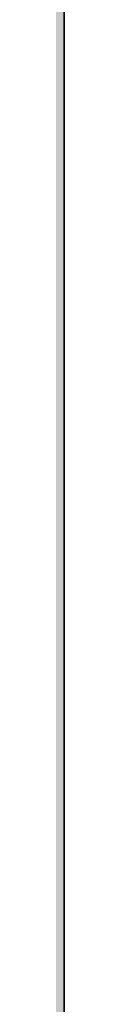
# Model space of a CAD drawing. Units: inches. Extents: x 2091 to 2899, y 967 to 2217.
# Tile 62 of 256: x 2212.1436 to 2212.1436, y 1100.1654 to 1100.4988. Entities that reach past the tile are written whole.
import ezdxf

# ---------------------------------------------------------------- set-up
doc = ezdxf.new("R2010")
doc.units = ezdxf.units.IN
doc.layers.add('A-WALL', color=7, linetype='Continuous', lineweight=35)
doc.layers.add('A-WALL-PATT', color=141, linetype='Continuous', lineweight=13, true_color=0xadddf7)

msp = doc.modelspace()

# ---------------------------------------------------------------- hatches: boundary and pattern name
at = {"layer": 'A-WALL-PATT'}
h = msp.add_hatch(color=256, dxfattribs=at)
h.dxf.hatch_style = 1
h.paths.add_polyline_path([(2212.1436, 1941.41906), (2387.6436, 1941.41906), (2387.6436, 1824.41906), (2392.1436, 1824.41906), (2392.1436, 1941.41906), (2609.6436, 1941.41906), (2609.6436, 1825.91906), (2614.1436, 1825.91906), (2614.1436, 1941.41906), (2794.1436, 1941.41906), (2794.1436, 1928.76217), (2803.1436, 1928.76217), (2803.1436, 2050.91906), (2203.1436, 2050.91906), (2203.1436, 1900.75786), (2212.1436, 1900.75786)])
h.paths.add_polyline_path([(2212.1436, 1945.91906), (2212.1436, 2041.91906), (2794.1436, 2041.91906), (2794.1436, 1945.91906), (2402.24824, 1945.91906), (2401.10243, 1945.77583), (2398.70243, 1945.77583)], flags=16)
h.paths.add_polyline_path([(2230.22986, 1948.06279), (2227.34986, 1949.50279), (2225.90986, 1951.90279), (2223.98986, 1952.86279), (2223.02986, 1955.26279), (2222.06986, 1959.58279), (2222.06986, 1963.42279), (2223.02986, 1965.66279), (2223.98986, 1965.34279), (2225.58591, 1963.86075), (2226.91153, 1964.95726), (2226.94886, 1965.93879), (2227.77832, 1966.95214), (2228.19992, 1968.8787), (2230.70986, 1964.86279), (2233.58986, 1966.30279), (2233.60731, 1966.33187), (2233.77266, 1964.9382), (2234.6338, 1963.67647), (2235.02986, 1963.90279), (2236.28203, 1965.57236), (2235.98986, 1962.94279), (2237.95451, 1957.54), (2238.38986, 1957.90279), (2239.21586, 1960.30579), (2238.65457, 1966.38496), (2238.69279, 1966.43807), (2238.84058, 1967.49971), (2238.78029, 1967.68749), (2238.88054, 1967.78676), (2238.66686, 1966.25179), (2239.21586, 1960.30579), (2238.38986, 1957.90279), (2236.94986, 1956.70279), (2234.54986, 1949.98279)], flags=0)
h.paths.add_polyline_path([(2278.01197, 1948.06279), (2276.49643, 1947.87335), (2275.84983, 1947.68861), (2274.65197, 1947.10279)], flags=0)
h.paths.add_polyline_path([(2269.85197, 1955.74279), (2268.27618, 1956.62933), (2270.8673, 1956.3484), (2269.37197, 1958.14279), (2268.71496, 1959.19233), (2270.56983, 1958.72861), (2268.58073, 1961.90609), (2270.81197, 1960.89188), (2270.81197, 1963.42279), (2271.39331, 1964.77926), (2270.29176, 1966.1562), (2271.77197, 1965.66279), (2272.14139, 1966.52476), (2273.92983, 1965.92861), (2275.63039, 1968.0543), (2276.33194, 1966.72186), (2276.52043, 1966.95214), (2276.94203, 1968.8787), (2277.73429, 1967.61108), (2278.13989, 1969.46452), (2279.65912, 1967.03374), (2280.41197, 1966.78279), (2280.9493, 1967.58879), (2281.60983, 1967.36861), (2282.13327, 1968.15376), (2282.34924, 1966.33344), (2282.34985, 1966.33259), (2283.40755, 1968.09542), (2283.71263, 1965.52402), (2284.32022, 1964.63379), (2284.51181, 1964.88924), (2284.23497, 1965.70479), (2284.50047, 1967.31896), (2284.90794, 1965.41742), (2285.39631, 1966.06858), (2285.43283, 1966.29061), (2285.47334, 1966.17128), (2286.35392, 1967.34539), (2286.22201, 1966.15817), (2287.66349, 1968.08015), (2287.71397, 1968.44279), (2288.4816, 1969.01668), (2288.57399, 1968.7289), (2288.91746, 1969.06904), (2288.60683, 1966.83761), (2288.92873, 1963.35131), (2288.93497, 1963.35679), (2288.92973, 1963.34042), (2289.01528, 1962.41387), (2290.11122, 1963.87513), (2290.13283, 1963.94261), (2290.21767, 1964.01706), (2290.11122, 1963.87513), (2289.15583, 1960.89161), (2288.59404, 1959.25723), (2288.57197, 1959.10279), (2289.53197, 1960.54279), (2290.01197, 1962.46279), (2290.19184, 1962.64266), (2289.76983, 1959.68861), (2286.88983, 1957.28861), (2284.48983, 1950.56861), (2283.31466, 1950.04631), (2283.29197, 1949.98279), (2280.29006, 1948.64861), (2281.12983, 1948.64861), (2282.56983, 1948.16861), (2283.20473, 1948.06279), (2278.97197, 1948.06279), (2276.09197, 1949.50279), (2274.65197, 1951.90279), (2272.73197, 1952.86279)], flags=0)
h.paths.add_polyline_path([(2271.15887, 1958.02177), (2272.96983, 1955.84861), (2272.00983, 1960.16861), (2272.00983, 1964.00861), (2272.62443, 1965.44266), (2274.32802, 1963.86075), (2275.65365, 1964.95726), (2275.63774, 1964.53909), (2277.41223, 1966.00689), (2277.03297, 1965.15679), (2276.82992, 1964.9756), (2276.76601, 1963.29501), (2277.44964, 1962.66022), (2279.45197, 1964.86279), (2282.33197, 1966.30279), (2283.52983, 1966.88861), (2283.29451, 1966.77095), (2283.91299, 1963.8847), (2284.89925, 1964.44827), (2284.73197, 1962.94279), (2286.69662, 1957.54), (2287.13197, 1957.90279), (2287.54191, 1959.09539), (2287.7794, 1958.44231), (2285.68274, 1956.6951), (2285.8765, 1959.79534), (2284.73197, 1962.94279), (2284.89925, 1964.44827), (2283.91299, 1963.8847), (2284.22383, 1962.43412), (2283.42436, 1963.60548), (2281.60983, 1962.56861), (2281.12983, 1960.16861), (2282.08983, 1956.32861), (2283.04983, 1952.96861), (2282.56983, 1950.56861), (2280.16983, 1948.64861), (2279.88332, 1948.79187), (2278.97197, 1948.06279), (2278.97197, 1949.02279), (2278.67231, 1949.39737), (2277.28983, 1950.08861), (2275.84983, 1952.48861), (2273.92983, 1953.44861), (2272.48983, 1954.88861), (2271.92165, 1954.88861), (2271.77197, 1955.26279)], flags=0)
h.paths.add_polyline_path([(2311.99415, 1955.74279), (2312.06272, 1955.67422), (2312.0551, 1955.7085)], flags=0)
h.paths.add_polyline_path([(2331.95615, 1963.95179), (2333.39615, 1965.39179), (2331.07715, 1963.35679), (2330.9986, 1963.11152)], flags=0)
h.paths.add_polyline_path([(2310.55415, 1954.30279), (2307.03981, 1956.27994), (2310.7629, 1955.87628), (2312.47415, 1953.82279), (2313.43415, 1951.42279), (2315.35415, 1950.46279), (2316.79415, 1948.06279), (2317.46615, 1947.72679), (2319.36869, 1947.96461), (2317.75415, 1949.98279), (2317.56953, 1950.61048), (2316.79415, 1951.90279), (2314.87415, 1952.86279), (2313.91415, 1955.26279), (2311.51415, 1958.14279), (2309.37549, 1961.55917), (2311.51415, 1960.33708), (2311.51415, 1961.98279), (2310.60467, 1963.11963), (2311.72661, 1962.47853), (2312.41833, 1964.09256), (2312.25596, 1964.29552), (2313.19415, 1963.98279), (2313.91415, 1965.66279), (2314.64678, 1965.41858), (2315.35415, 1966.30279), (2316.79415, 1967.74279), (2316.15744, 1966.9469), (2317.03411, 1965.28186), (2317.2226, 1965.51214), (2317.77705, 1968.04577), (2318.47411, 1966.72186), (2318.6626, 1966.95214), (2319.0842, 1968.8787), (2321.20705, 1965.48215), (2322.16142, 1966.9137), (2322.55415, 1966.78279), (2322.78599, 1967.13056), (2322.88165, 1966.32429), (2323.31204, 1965.72174), (2323.65129, 1965.89136), (2324.3965, 1967.13338), (2324.65694, 1964.9382), (2324.97199, 1964.47661), (2325.38728, 1967.0015), (2325.94081, 1964.41835), (2327.22893, 1966.13584), (2327.16632, 1965.57236), (2328.05914, 1966.76278), (2328.22458, 1966.24749), (2329.66797, 1967.67691), (2329.66458, 1967.68749), (2329.76482, 1967.78676), (2329.55115, 1966.25179), (2330.10015, 1960.30579), (2329.33281, 1958.07347), (2329.31306, 1957.93523), (2329.63415, 1958.20279), (2330.23415, 1959.10279), (2330.71415, 1961.02279), (2331.03415, 1961.34279), (2330.71415, 1959.10279), (2329.63415, 1958.20279), (2329.27415, 1957.66279), (2327.71211, 1956.3611), (2325.43415, 1949.98279), (2324.33377, 1949.49374), (2323.99415, 1948.54279), (2319.67415, 1946.62279), (2316.79415, 1948.06279), (2315.35415, 1950.46279), (2313.43415, 1951.42279)], flags=0)
h.paths.add_polyline_path([(2321.33568, 1947.95202), (2321.11415, 1948.06279), (2321.11415, 1949.02279), (2319.19415, 1951.42279), (2316.79415, 1959.58279), (2316.66324, 1959.58279), (2315.35415, 1958.14279), (2314.39415, 1958.14279), (2313.1483, 1958.70908), (2312.95415, 1959.58279), (2312.95415, 1960.89188), (2315.83415, 1959.58279), (2316.66324, 1959.58279), (2317.31471, 1960.29941), (2315.0302, 1962.42075), (2316.35582, 1963.51726), (2316.37234, 1963.95162), (2316.4702, 1963.86075), (2317.79582, 1964.95726), (2317.75522, 1963.88969), (2319.17515, 1965.15679), (2319.49841, 1965.88137), (2321.11415, 1965.34279), (2323.23589, 1962.37236), (2325.68635, 1963.77262), (2325.54279, 1962.48058), (2325.19878, 1963.49401), (2324.47851, 1963.08243), (2324.92601, 1960.99412), (2324.07809, 1962.23647), (2322.41479, 1961.28602), (2322.07415, 1959.58279), (2323.03415, 1955.74279), (2323.99415, 1952.38279), (2323.51415, 1949.98279), (2322.14272, 1948.88565), (2322.07415, 1948.54279)], flags=0)
h.paths.add_polyline_path([(2320.20748, 1963.33746), (2320.15415, 1963.42279), (2320.39415, 1963.54279)], flags=0)
h.paths.add_polyline_path([(2353.85053, 1965.8105), (2354.03053, 1965.7505), (2354.33053, 1966.4505), (2354.33053, 1966.9305)], flags=0)
h.paths.add_polyline_path([(2359.02058, 1969.02641), (2359.09838, 1968.90193), (2359.23353, 1969.5195), (2359.23353, 1969.9995)], flags=0)
h.paths.add_polyline_path([(2358.25669, 1966.68167), (2357.9836, 1966.34803), (2358.21127, 1966.14617), (2358.41049, 1966.38957)], flags=0)
h.paths.add_polyline_path([(2357.76847, 1966.05878), (2357.7322, 1965.10497), (2357.75105, 1965.12056), (2357.76953, 1965.6065), (2357.76953, 1966.05784)], flags=0)
h.paths.add_polyline_path([(2359.11153, 1965.3045), (2359.11153, 1964.8245), (2359.84453, 1966.4675), (2359.84453, 1966.9475)], flags=0)
h.paths.add_polyline_path([(2360.22368, 1966.62145), (2360.69853, 1969.3625), (2360.69853, 1969.8425), (2360.21053, 1967.0255), (2360.21053, 1966.6425)], flags=0)
h.paths.add_polyline_path([(2363.45053, 1967.8905), (2363.45053, 1968.3705), (2362.49053, 1966.9305), (2362.65604, 1966.69878)], flags=0)
h.paths.add_polyline_path([(2364.47552, 1966.07883), (2365.85053, 1968.3705), (2365.85053, 1968.8505), (2364.42798, 1966.47958)], flags=0)
h.paths.add_polyline_path([(2366.31353, 1965.8525), (2366.36671, 1965.69583), (2366.80253, 1968.3455), (2366.80253, 1968.8255)], flags=0)
h.paths.add_polyline_path([(2367.16531, 1965.80354), (2367.29053, 1966.9305), (2367.29053, 1967.4105), (2367.1027, 1965.72007)], flags=0)
h.paths.add_polyline_path([(2370.03653, 1959.9735), (2371.01353, 1963.0245), (2371.01353, 1963.5045), (2370.03653, 1960.4535)], flags=0)
h.paths.add_polyline_path([(2371.61053, 1960.2105), (2372.57053, 1961.6505), (2372.57053, 1962.1305), (2371.80253, 1960.9785)], flags=0)
h.paths.add_polyline_path([(2350.87367, 1956.00509), (2351.93053, 1955.8905), (2354.49053, 1953.3305), (2353.85053, 1954.9305), (2351.45053, 1957.8105), (2347.93553, 1963.4255), (2347.93553, 1963.9055), (2351.45053, 1958.2905), (2353.70507, 1955.58505), (2352.89053, 1959.2505), (2352.89053, 1959.7305), (2352.89053, 1961.92479), (2356.73053, 1959.7305), (2358.45447, 1961.62684), (2354.81053, 1965.0105), (2355.03086, 1965.28591), (2358.69109, 1961.88712), (2361.53053, 1965.0105), (2364.3765, 1966.43348), (2364.52439, 1965.18691), (2365.45447, 1963.82418), (2365.88107, 1964.06795), (2365.37053, 1966.4505), (2365.37053, 1966.9305), (2366.81053, 1960.2105), (2366.81053, 1959.7305), (2366.38871, 1952.98141), (2367.77053, 1956.8505), (2368.64123, 1957.57608), (2366.81053, 1962.6105), (2366.81053, 1963.0905), (2368.77518, 1957.68771), (2369.21053, 1958.0505), (2370.00159, 1960.35187), (2369.47523, 1966.05267), (2369.51346, 1966.10578), (2369.51417, 1966.11091), (2369.47523, 1966.53267), (2369.51346, 1966.58578), (2369.61463, 1967.31259), (2369.18253, 1968.6585), (2369.18253, 1969.1385), (2369.60096, 1967.83519), (2369.7012, 1967.93447), (2369.71795, 1968.05474), (2370.14518, 1968.37414), (2369.77871, 1968.01122), (2369.7012, 1967.45447), (2370.46816, 1968.214), (2369.67494, 1967.26577), (2369.51417, 1966.11091), (2370.03653, 1960.4535), (2370.03653, 1959.9735), (2369.44176, 1958.24319), (2370.65053, 1959.2505), (2371.04582, 1962.01756), (2371.13053, 1962.1305), (2370.65053, 1958.7705), (2367.77053, 1956.3705), (2365.37053, 1949.6505), (2362.0791, 1948.18764), (2363.45053, 1947.7305), (2361.05053, 1947.7305), (2360.09053, 1947.7305), (2357.10386, 1947.35717), (2360.09053, 1948.2105), (2358.17053, 1949.1705), (2356.73053, 1951.5705), (2354.81053, 1952.5305), (2351.93053, 1955.4105)], flags=0)
h.paths.add_polyline_path([(2361.05053, 1948.6905), (2359.13053, 1951.0905), (2356.73053, 1959.2505), (2355.77053, 1959.2505), (2352.89053, 1960.55959), (2352.89053, 1961.44479), (2355.89053, 1959.7305), (2356.73053, 1959.7305), (2356.83719, 1959.36783), (2361.53053, 1964.5305), (2363.24842, 1965.38945), (2364.92531, 1963.0418), (2362.49053, 1961.6505), (2362.06386, 1959.51717), (2362.97053, 1955.8905), (2363.93053, 1952.5305), (2363.93053, 1952.0505), (2363.45053, 1949.6505), (2361.05053, 1947.7305)], flags=0)
h.paths.add_polyline_path([(2359.13053, 1951.5705), (2359.29053, 1951.3705), (2361.05053, 1954.4505), (2361.05053, 1954.9305)], flags=0)
h.paths.add_polyline_path([(2357.21953, 1966.5455), (2356.79253, 1968.8145), (2356.79253, 1969.2945), (2357.21953, 1967.0255)], flags=0)
h.paths.add_polyline_path([(2361.05053, 1954.4505), (2361.53053, 1958.7705), (2361.53053, 1959.2505), (2361.05053, 1954.9305)], flags=0)
h.paths.add_polyline_path([(2402.54829, 1948.48608), (2402.30243, 1948.41583), (2402.59043, 1948.41583)], flags=0)
h.paths.add_polyline_path([(2394.14243, 1956.09583), (2395.68505, 1954.55321), (2396.7205, 1953.97068), (2396.06243, 1955.61583), (2395.24138, 1956.6011), (2395.8789, 1956.44171), (2395.10243, 1959.93583), (2395.10243, 1963.77583), (2396.06243, 1966.01583), (2397.02243, 1965.69583), (2398.61848, 1964.21379), (2399.94411, 1965.3103), (2399.98143, 1966.29183), (2400.81089, 1967.30518), (2401.23249, 1969.23174), (2403.53795, 1965.54301), (2403.94198, 1967.38932), (2404.70243, 1967.13583), (2405.46033, 1966.07478), (2406.62243, 1966.65583), (2406.63988, 1966.68491), (2406.80523, 1965.29124), (2406.92569, 1965.11475), (2407.34243, 1964.97583), (2407.87433, 1965.77367), (2408.1691, 1964.39805), (2409.31461, 1965.9254), (2409.21746, 1965.05105), (2409.44523, 1963.13124), (2410.30637, 1961.86951), (2410.70243, 1962.09583), (2411.44227, 1963.08228), (2411.16543, 1963.89783), (2411.61643, 1966.63976), (2411.72536, 1966.79111), (2411.87315, 1967.85275), (2411.81286, 1968.04053), (2411.91311, 1968.1398), (2411.69943, 1966.60483), (2412.24843, 1960.65883), (2413.22543, 1963.70983), (2414.3779, 1964.72116), (2414.51315, 1965.69275), (2414.45286, 1965.88053), (2414.55311, 1965.9798), (2414.3779, 1964.72116), (2414.51982, 1964.8457), (2414.36536, 1964.63111), (2414.33943, 1964.44483), (2414.88843, 1958.49883), (2414.06243, 1956.09583), (2412.62243, 1954.89583), (2410.17137, 1948.03285), (2410.01672, 1948.0844), (2405.90243, 1946.25583), (2405.90243, 1947.21583), (2405.20425, 1948.08856), (2404.22243, 1948.41583), (2403.26243, 1948.41583), (2400.38243, 1949.85583), (2399.66243, 1951.05583), (2397.98243, 1952.73583), (2397.02243, 1953.21583), (2395.68505, 1954.55321), (2392.65678, 1956.25691)], flags=0)
h.paths.add_polyline_path([(2409.08565, 1964.40744), (2409.13036, 1964.27572), (2409.26243, 1964.49583)], flags=0)
h.paths.add_polyline_path([(2397.74243, 1961.61583), (2398.70243, 1963.85583), (2399.66243, 1963.53583), (2401.42656, 1965.74099), (2401.79142, 1966.5588), (2402.07143, 1965.07083), (2402.83551, 1964.39337), (2403.2624, 1964.9149), (2403.33812, 1964.77109), (2402.61552, 1963.97622), (2402.49861, 1960.90224), (2403.543, 1959.93245), (2404.4132, 1960.88968), (2404.70243, 1962.33583), (2407.91635, 1964.17235), (2409.52021, 1961.92694), (2410.98708, 1957.89304), (2411.42243, 1958.25583), (2412.04796, 1960.07562), (2412.41034, 1959.07909), (2411.67562, 1958.46682), (2411.66243, 1958.25583), (2411.62607, 1958.42553), (2409.98243, 1957.05583), (2407.58243, 1950.33583), (2403.26243, 1948.41583), (2403.26243, 1949.37583), (2401.34243, 1951.77583), (2399.41651, 1958.32398), (2397.74243, 1959.08492), (2397.74243, 1959.97012), (2397.10243, 1960.33583), (2397.74243, 1960.04492)], flags=0)
h.paths.add_polyline_path([(2405.90243, 1952.97583), (2405.95043, 1953.40783), (2406.01672, 1953.17583)], flags=0)
h.paths.add_polyline_path([(2449.81778, 1967.11401), (2449.75232, 1967.13583), (2449.7937, 1967.0779)], flags=0)
h.paths.add_polyline_path([(2451.6977, 1966.61812), (2451.74089, 1966.69012), (2451.69205, 1966.6657)], flags=0)
h.paths.add_polyline_path([(2454.34363, 1965.73757), (2455.75232, 1967.61583), (2455.99232, 1968.09583), (2454.3645, 1965.9254)], flags=0)
h.paths.add_polyline_path([(2457.54732, 1968.86383), (2457.78732, 1969.34383), (2457.05432, 1968.79583), (2457.00762, 1968.46034)], flags=0)
h.paths.add_polyline_path([(2456.92178, 1967.85666), (2456.80224, 1968.22902), (2456.723, 1967.6598)], flags=0)
h.paths.add_polyline_path([(2457.30232, 1967.37683), (2457.54232, 1967.85683), (2456.81032, 1966.83983), (2456.74052, 1966.70022), (2456.74902, 1966.60811)], flags=0)
h.paths.add_polyline_path([(2458.27532, 1963.70983), (2458.15534, 1963.33515), (2460.35432, 1965.26483), (2460.59432, 1965.74483)], flags=0)
h.paths.add_polyline_path([(2458.39232, 1962.81583), (2458.36409, 1962.61819), (2459.59232, 1964.25583), (2459.83232, 1964.73583)], flags=0)
h.paths.add_polyline_path([(2459.35232, 1962.81583), (2459.27232, 1962.49583), (2460.07232, 1963.29583), (2460.31232, 1963.77583)], flags=0)
h.paths.add_polyline_path([(2458.68032, 1960.60783), (2458.63232, 1960.41583), (2459.59232, 1961.85583), (2459.83232, 1962.33583)], flags=0)
h.paths.add_polyline_path([(2437.83817, 1956.24265), (2439.19232, 1956.09583), (2441.35232, 1953.93583), (2440.87232, 1955.13583), (2438.47232, 1958.01583), (2438.07156, 1958.65602), (2438.71232, 1958.49583), (2440.6396, 1956.18311), (2439.91232, 1959.45583), (2439.91232, 1963.29583), (2441.35232, 1966.65583), (2441.59232, 1967.13583), (2441.11232, 1966.01583), (2442.07232, 1965.69583), (2443.98899, 1968.09167), (2444.24132, 1966.75083), (2444.9168, 1966.15192), (2445.67657, 1967.08014), (2446.25532, 1969.72483), (2446.49532, 1970.20483), (2446.28238, 1969.23174), (2447.36267, 1967.50327), (2447.72032, 1969.56783), (2447.96032, 1970.04783), (2447.48548, 1967.30678), (2448.79232, 1965.21583), (2448.47232, 1964.86383), (2448.55232, 1964.73583), (2451.45205, 1966.1857), (2451.61512, 1964.81124), (2452.30792, 1963.79617), (2453.23451, 1964.32565), (2454.07232, 1960.41583), (2453.62869, 1953.31765), (2454.79232, 1956.57583), (2455.03232, 1957.05583), (2455.71884, 1957.62793), (2453.83232, 1962.81583), (2453.94097, 1963.79362), (2453.33532, 1965.57783), (2453.82432, 1968.55083), (2454.06432, 1969.03083), (2453.57532, 1966.05783), (2454.04033, 1964.68792), (2453.83232, 1962.81583), (2455.71884, 1957.62793), (2456.36721, 1958.16824), (2457.05832, 1960.17883), (2457.29832, 1960.65883), (2456.47232, 1958.25583), (2457.71773, 1959.29367), (2457.67232, 1958.97583), (2454.88995, 1956.65719), (2453.61414, 1953.08492), (2453.59232, 1952.73583), (2453.35232, 1952.25583), (2453.3596, 1952.3722), (2452.63232, 1950.33583), (2452.39232, 1949.85583), (2449.20375, 1948.43869), (2450.71232, 1947.93583), (2448.07232, 1947.93583), (2447.11232, 1947.93583), (2444.55232, 1947.61583), (2447.1996, 1948.3722), (2445.19232, 1949.37583), (2443.75232, 1951.77583), (2441.83232, 1952.73583), (2438.95232, 1955.61583)], flags=0)
h.paths.add_polyline_path([(2443.99232, 1959.93583), (2444.04032, 1959.77263), (2444.12155, 1959.86199)], flags=0)
h.paths.add_polyline_path([(2442.91232, 1959.93583), (2443.03232, 1959.93583), (2442.44566, 1960.2025)], flags=0)
h.paths.add_polyline_path([(2444.98294, 1965.01968), (2445.27932, 1965.26483), (2445.51932, 1965.74483), (2444.994, 1965.3103)], flags=0)
h.paths.add_polyline_path([(2446.13332, 1965.02983), (2446.33037, 1965.4715), (2444.97032, 1964.25783), (2444.73032, 1963.77783)], flags=0)
h.paths.add_polyline_path([(2442.79232, 1959.45583), (2443.75232, 1959.45583), (2446.15232, 1951.29583), (2446.41232, 1951.75083), (2446.39232, 1951.77583), (2448.0806, 1954.73032), (2448.55232, 1958.97583), (2441.83232, 1965.21583), (2442.15495, 1965.61911), (2448.79232, 1959.45583), (2448.31232, 1955.13583), (2448.07232, 1954.65583), (2446.41232, 1951.75083), (2448.31232, 1949.37583), (2448.31232, 1948.41583), (2450.54089, 1950.19869), (2450.95232, 1952.25583), (2449.99232, 1955.61583), (2449.03232, 1959.45583), (2449.51232, 1961.85583), (2449.75232, 1962.33583), (2449.6749, 1961.94874), (2452.99451, 1963.84565), (2453.06441, 1963.51941), (2452.88461, 1963.78285), (2449.6749, 1961.94874), (2449.27232, 1959.93583), (2450.23232, 1956.09583), (2451.19232, 1952.73583), (2450.71232, 1950.33583), (2450.47232, 1949.85583), (2448.07232, 1947.93583), (2448.07232, 1948.53583), (2445.43232, 1949.85583), (2443.99232, 1952.25583), (2442.07232, 1953.21583), (2441.11232, 1955.61583), (2440.15232, 1959.93583), (2440.15232, 1960.65583)], flags=0)
h.paths.add_polyline_path([(2456.69232, 1966.98583), (2457.60832, 1968.08083), (2457.84832, 1968.56083), (2456.93232, 1967.46583)], flags=0)
h.paths.add_polyline_path([(2489.89657, 1966.58024), (2489.94295, 1966.18935), (2490.74749, 1967.53025), (2491.31912, 1968.95116)], flags=0)
h.paths.add_polyline_path([(2473.56247, 1956.40713), (2477.13998, 1956.01926), (2476.95533, 1956.24083), (2475.10805, 1957.28011), (2476.34749, 1956.97025), (2475.1869, 1958.82422), (2476.91912, 1958.39116), (2475.41164, 1960.79927), (2477.78749, 1959.71934), (2477.78749, 1962.25025), (2477.6374, 1962.43786), (2477.82255, 1962.33206), (2478.35912, 1963.58406), (2478.35912, 1963.67116), (2477.32435, 1964.96463), (2478.71483, 1964.50114), (2479.31912, 1965.91116), (2480.27912, 1965.59116), (2481.78397, 1967.47221), (2482.11649, 1965.70525), (2482.88056, 1965.02778), (2483.20931, 1965.42941), (2483.22017, 1965.71509), (2483.07594, 1965.98902), (2483.71176, 1966.76581), (2484.13049, 1968.67925), (2484.70212, 1970.10016), (2484.48918, 1969.12707), (2486.5029, 1965.90511), (2487.38749, 1965.61025), (2488.15342, 1966.75914), (2488.71702, 1965.97011), (2489.20009, 1966.21164), (2489.33067, 1965.11099), (2490.3939, 1963.62246), (2490.66077, 1963.77496), (2490.49391, 1964.55364), (2490.92306, 1963.92484), (2491.31912, 1964.15116), (2491.33339, 1964.17018), (2491.21049, 1964.53225), (2491.28176, 1964.96554), (2491.42579, 1964.29338), (2494.07648, 1967.82763), (2494.49792, 1966.51494), (2494.59817, 1966.61422), (2494.68949, 1967.27025), (2495.10675, 1967.5822), (2495.12984, 1967.74807), (2495.06955, 1967.93585), (2495.1698, 1968.03513), (2495.03178, 1967.04363), (2495.75382, 1967.75868), (2494.98205, 1966.68644), (2494.95612, 1966.50016), (2495.47902, 1960.83685), (2495.91049, 1962.18425), (2496.48212, 1963.60516), (2496.07269, 1962.32659), (2496.7689, 1962.93754), (2496.59912, 1962.71116), (2496.11912, 1959.35116), (2496.73287, 1960.27179), (2496.98749, 1961.29025), (2497.55912, 1962.71116), (2497.07912, 1960.79116), (2496.50749, 1959.37025), (2495.54749, 1957.93025), (2492.75884, 1955.60638), (2490.83912, 1950.23116), (2490.26749, 1948.81025), (2485.94749, 1946.89025), (2483.06749, 1948.33025), (2481.62749, 1950.73025), (2479.70749, 1951.69025), (2476.82749, 1954.57025)], flags=0)
h.paths.add_polyline_path([(2485.57697, 1948.31339), (2485.55912, 1948.31116), (2485.57876, 1948.31116)], flags=0)
h.paths.add_polyline_path([(2478.64506, 1954.55116), (2478.10904, 1956.96326), (2479.31912, 1955.51116), (2480.27912, 1953.11116), (2482.19912, 1952.15116), (2483.63912, 1949.75116), (2486.51912, 1948.31116), (2486.51912, 1949.27116), (2484.73931, 1951.49593), (2484.02749, 1950.25025), (2481.62749, 1958.41025), (2482.37515, 1959.23267), (2482.19912, 1959.83116), (2483.19757, 1960.92946), (2479.70749, 1964.17025), (2480.60336, 1965.29008), (2481.87517, 1964.10911), (2482.66639, 1964.76358), (2482.61536, 1963.4218), (2482.9892, 1963.07466), (2484.00849, 1963.98425), (2484.68361, 1965.49751), (2484.58012, 1965.40516), (2485.35727, 1967.14711), (2485.12065, 1965.7812), (2486.42749, 1963.69025), (2488.14538, 1964.5492), (2489.82227, 1962.20155), (2490.74749, 1962.73025), (2491.99966, 1964.39981), (2492.07605, 1965.08726), (2492.21289, 1964.68412), (2492.48537, 1965.04743), (2492.27912, 1963.19116), (2494.24377, 1957.78837), (2494.5625, 1958.05398), (2494.93349, 1959.13325), (2495.50512, 1960.55416), (2494.67912, 1958.15116), (2494.10749, 1956.73025), (2494.5625, 1958.05398), (2493.40854, 1957.09235), (2491.70749, 1961.77025), (2491.99966, 1964.39981), (2490.74749, 1962.73025), (2487.71203, 1960.9957), (2487.47912, 1959.83116), (2488.43912, 1955.99116), (2489.39912, 1952.63116), (2488.91912, 1950.23116), (2488.57692, 1949.9574), (2488.34749, 1948.81025), (2487.65172, 1948.25363), (2487.47912, 1948.31116), (2486.51912, 1948.31116), (2483.63912, 1949.75116), (2482.19912, 1952.15116), (2480.27912, 1953.11116), (2478.83912, 1954.55116)], flags=0)
h.paths.add_polyline_path([(2526.64825, 1966.98752), (2526.51734, 1967.03116), (2526.6001, 1966.9153)], flags=0)
h.paths.add_polyline_path([(2528.47064, 1966.44666), (2528.57449, 1966.61973), (2528.45707, 1966.56102)], flags=0)
h.paths.add_polyline_path([(2534.13334, 1967.49616), (2534.15669, 1967.54285), (2534.05984, 1967.4083)], flags=0)
h.paths.add_polyline_path([(2536.16192, 1964.0506), (2535.15734, 1962.71116), (2535.10087, 1962.31587), (2536.11734, 1963.67116), (2536.42053, 1964.27754)], flags=0)
h.paths.add_polyline_path([(2535.15734, 1959.83116), (2536.11734, 1961.27116), (2536.59734, 1962.23116), (2535.25334, 1960.21516)], flags=0)
h.paths.add_polyline_path([(2513.24904, 1956.2848), (2516.22118, 1955.96256), (2514.99734, 1957.43116), (2514.19582, 1958.71154), (2515.47734, 1958.39116), (2516.93189, 1956.64571), (2516.43734, 1958.87116), (2516.43734, 1962.71116), (2516.87269, 1963.72697), (2515.34643, 1965.6348), (2517.39734, 1964.95116), (2517.87734, 1966.07116), (2518.35734, 1967.03116), (2517.87734, 1965.91116), (2518.83734, 1965.59116), (2520.48659, 1967.65272), (2520.76634, 1966.16616), (2521.53042, 1965.48869), (2521.78144, 1965.79537), (2521.80091, 1966.30727), (2521.4778, 1966.92094), (2521.24634, 1967.12616), (2521.1777, 1967.49091), (2521.4778, 1966.92094), (2522.01042, 1966.44869), (2522.25739, 1966.75042), (2522.78034, 1969.14016), (2523.26034, 1970.10016), (2523.0474, 1969.12707), (2524.67313, 1966.5259), (2526.03734, 1966.07116), (2526.79524, 1965.01011), (2527.97707, 1965.60102), (2528.14014, 1964.22657), (2528.66459, 1963.45816), (2529.38862, 1963.87189), (2529.32967, 1964.14699), (2529.48128, 1963.92484), (2529.87734, 1964.15116), (2529.98401, 1964.29338), (2529.78905, 1965.20318), (2530.0624, 1964.3979), (2532.80248, 1968.05135), (2533.14777, 1966.97585), (2533.24802, 1967.07513), (2533.33934, 1967.73116), (2533.67285, 1967.98049), (2533.72802, 1968.03513), (2533.51434, 1966.50016), (2534.02472, 1960.9725), (2534.56034, 1962.64516), (2535.04034, 1963.60516), (2534.06334, 1960.55416), (2533.23734, 1958.15116), (2534.28815, 1959.02684), (2534.19734, 1958.39116), (2531.5126, 1956.15387), (2529.39734, 1950.23116), (2528.91734, 1949.27116), (2526.44877, 1948.17402), (2527.47734, 1947.83116), (2530.35734, 1947.35116), (2524.59734, 1947.35116), (2521.71734, 1948.79116), (2520.27734, 1951.19116), (2518.35734, 1952.15116), (2515.47734, 1955.03116)], flags=0)
h.paths.add_polyline_path([(2523.93476, 1967.19031), (2523.61951, 1966.48369), (2523.7705, 1966.24211)], flags=0)
h.paths.add_polyline_path([(2518.83734, 1953.11116), (2517.87734, 1955.51116), (2516.88498, 1959.97678), (2516.91734, 1959.96207), (2516.91734, 1962.02545), (2520.75734, 1959.83116), (2522.02495, 1961.22553), (2518.35734, 1964.63116), (2519.00259, 1965.43772), (2520.43339, 1964.10911), (2521.30112, 1964.82687), (2521.24516, 1963.35533), (2525.63831, 1959.27598), (2526.03734, 1961.27116), (2529.39734, 1963.19116), (2530.64952, 1964.86073), (2530.66472, 1964.99755), (2530.69196, 1964.91731), (2531.08778, 1965.44507), (2530.94599, 1964.16894), (2530.69196, 1964.91731), (2529.39734, 1963.19116), (2526.3625, 1961.45697), (2526.03734, 1959.83116), (2526.99734, 1955.99116), (2527.95734, 1952.63116), (2527.47734, 1950.23116), (2527.13449, 1949.95687), (2526.97393, 1949.15409), (2526.69734, 1949.03116), (2524.59734, 1947.35116), (2524.59734, 1948.31116), (2524.27734, 1948.71116), (2522.19734, 1949.75116), (2520.75734, 1952.15116)], flags=0)
h.paths.add_polyline_path([(2520.27734, 1958.87116), (2520.85334, 1959.50476), (2523.15734, 1951.67116), (2524.61389, 1954.22013), (2524.59734, 1954.07116), (2522.67734, 1950.71116)], flags=0)
h.paths.add_polyline_path([(2559.37091, 1966.31116), (2559.39841, 1966.32491), (2559.40194, 1966.3453)], flags=0)
h.paths.add_polyline_path([(2549.77091, 1957.19116), (2552.65091, 1954.31116), (2552.13399, 1955.60347), (2550.61091, 1957.43116), (2547.09591, 1963.04616), (2545.77591, 1965.20616), (2549.29091, 1959.59116), (2551.69091, 1956.71116), (2550.79293, 1960.75206), (2550.73091, 1960.78025), (2550.73091, 1964.87116), (2551.69091, 1967.11116), (2552.65091, 1966.79116), (2554.24696, 1965.30911), (2555.03425, 1965.96034), (2555.58167, 1966.64461), (2555.60991, 1967.38716), (2556.43937, 1968.40051), (2556.86097, 1970.32707), (2559.37091, 1966.31116), (2560.69091, 1964.15116), (2562.40881, 1965.01011), (2561.65091, 1966.07116), (2560.33091, 1968.23116), (2561.7585, 1966.23254), (2562.34721, 1967.11561), (2562.43371, 1966.38657), (2563.1278, 1965.3696), (2563.57091, 1965.59116), (2563.58836, 1965.62024), (2563.36254, 1967.52354), (2563.72249, 1965.84379), (2565.06, 1968.07298), (2564.73286, 1965.12872), (2565.11758, 1963.33338), (2567.44462, 1966.43611), (2567.31561, 1967.83333), (2567.35384, 1967.88644), (2567.50163, 1968.94807), (2567.44134, 1969.13585), (2567.54159, 1969.23513), (2567.32791, 1967.70016), (2567.87691, 1961.75416), (2568.74669, 1964.47033), (2568.63561, 1965.67333), (2568.67384, 1965.72644), (2568.82163, 1966.78807), (2568.76134, 1966.97585), (2568.86159, 1967.07513), (2568.64791, 1965.54016), (2568.72613, 1964.69303), (2568.85391, 1964.80516), (2568.74669, 1964.47033), (2568.81724, 1963.70626), (2568.97091, 1963.91116), (2568.86607, 1963.17731), (2569.19691, 1959.59416), (2568.37091, 1957.19116), (2566.93091, 1955.99116), (2564.62027, 1949.52137), (2564.65091, 1949.51116), (2564.61662, 1949.51116), (2564.53091, 1949.27116), (2560.21091, 1947.35116), (2557.33091, 1948.79116), (2556.0452, 1950.93402), (2556.01091, 1950.95116), (2555.85662, 1951.2083), (2553.97091, 1952.15116), (2551.09091, 1955.03116), (2546.65014, 1957.52951)], flags=0)
h.paths.add_polyline_path([(2567.02579, 1959.33023), (2567.03501, 1959.30489), (2567.05091, 1959.35116)], flags=0)
h.paths.add_polyline_path([(2551.96829, 1962.51837), (2553.01091, 1964.95116), (2553.97091, 1964.63116), (2555.56696, 1963.14911), (2556.89258, 1964.24563), (2556.92991, 1965.22716), (2557.14398, 1965.48869), (2556.42007, 1966.13056), (2556.39142, 1966.10499), (2556.37991, 1966.16616), (2556.42007, 1966.13056), (2556.95191, 1966.60516), (2557.09214, 1966.91948), (2557.57087, 1966.01023), (2557.75937, 1966.24051), (2557.41791, 1964.68016), (2556.89258, 1964.24563), (2556.80709, 1961.99757), (2560.69091, 1958.39116), (2560.63553, 1957.8927), (2560.81091, 1957.19116), (2561.77091, 1953.83116), (2561.29091, 1951.43116), (2559.11042, 1949.68677), (2559.15648, 1949.62919), (2563.02652, 1951.34921), (2562.61091, 1949.27116), (2560.21091, 1947.35116), (2560.21091, 1948.31116), (2559.25091, 1949.51116), (2558.89091, 1949.51116), (2558.89091, 1949.96116), (2558.29091, 1950.71116), (2558.0537, 1951.51767), (2556.97091, 1952.87116), (2555.06788, 1959.34146), (2552.05091, 1961.06545), (2552.05091, 1962.47116)], flags=0)
h.paths.add_polyline_path([(2588.33005, 1958.39116), (2588.61025, 1958.11096), (2588.55336, 1958.36695)], flags=0)
h.paths.add_polyline_path([(2594.74545, 1950.49309), (2593.95753, 1953.17202), (2593.13005, 1954.55116), (2591.21005, 1955.51116), (2590.25005, 1957.91116), (2588.30903, 1960.24038), (2586.17731, 1961.20935), (2587.85005, 1960.79116), (2587.25342, 1961.74425), (2588.44131, 1961.06545), (2588.44131, 1962.65553), (2588.42168, 1962.66535), (2588.44131, 1962.71116), (2586.91404, 1964.62026), (2588.87709, 1963.72796), (2589.29005, 1964.69154), (2589.29005, 1966.07116), (2590.25005, 1968.31116), (2591.21005, 1967.99116), (2592.8061, 1966.50911), (2594.13172, 1967.60563), (2594.16905, 1968.58716), (2594.99851, 1969.60051), (2595.4201, 1971.52707), (2597.93005, 1967.51116), (2600.81005, 1968.95116), (2600.8275, 1968.98024), (2600.99285, 1967.58657), (2601.85399, 1966.32484), (2602.10714, 1966.4695), (2602.23635, 1967.25507), (2602.35672, 1966.69338), (2603.50222, 1968.22073), (2603.21005, 1965.59116), (2605.1747, 1960.18837), (2605.50689, 1960.4652), (2605.02602, 1965.67333), (2605.06425, 1965.72644), (2605.21203, 1966.78807), (2605.15174, 1966.97585), (2605.25199, 1967.07513), (2605.34331, 1967.73116), (2605.9529, 1968.1869), (2605.87475, 1969.03333), (2605.91298, 1969.08644), (2606.06077, 1970.14807), (2606.00048, 1970.33585), (2606.10073, 1970.43513), (2605.88705, 1968.90016), (2606.43605, 1962.95416), (2605.61005, 1960.55116), (2605.99704, 1960.87365), (2606.56431, 1962.64516), (2608.24149, 1964.11694), (2608.01005, 1963.19116), (2607.05005, 1961.75116), (2606.63149, 1961.40236), (2606.20131, 1958.39116), (2603.32131, 1955.99116), (2600.92131, 1949.27116), (2596.60131, 1947.35116), (2593.72131, 1948.79116), (2592.85731, 1950.23116), (2592.65005, 1950.23116)], flags=0)
h.paths.add_polyline_path([(2596.60131, 1947.35116), (2596.60131, 1948.31116), (2594.68131, 1950.71116), (2596.15495, 1953.29003), (2595.53005, 1954.07116), (2593.19923, 1961.99596), (2592.65134, 1962.50471), (2591.78015, 1963.00253), (2593.28299, 1964.24563), (2593.32031, 1965.22716), (2594.14977, 1966.24051), (2594.57137, 1968.16707), (2596.18265, 1965.58902), (2596.95127, 1966.43451), (2598.04131, 1966.07116), (2598.79921, 1965.01011), (2599.96131, 1965.59116), (2599.97876, 1965.62024), (2600.14411, 1964.22657), (2601.00526, 1962.96484), (2601.40131, 1963.19116), (2602.65349, 1964.86073), (2602.36131, 1962.23116), (2603.79275, 1958.29472), (2601.97764, 1953.21243), (2601.94621, 1952.70945), (2599.46876, 1951.60836), (2599.00131, 1949.27116)], flags=0)
h.paths.add_polyline_path([(2597.56131, 1958.87116), (2597.67097, 1959.41942), (2597.59505, 1958.7362)], flags=0)
h.paths.add_polyline_path([(2623.6663, 1961.25438), (2625.51916, 1960.79116), (2624.96554, 1961.67553), (2627.19916, 1960.66025), (2627.19916, 1961.15116), (2626.95916, 1962.23116), (2626.95916, 1963.49116), (2625.58232, 1965.21221), (2626.95916, 1964.42545), (2626.95916, 1965.83116), (2626.86916, 1965.86116), (2627.91916, 1968.31116), (2628.87916, 1967.99116), (2630.47521, 1966.50911), (2631.80084, 1967.60563), (2631.83816, 1968.58716), (2632.66762, 1969.60051), (2633.08922, 1971.52707), (2635.59916, 1967.51116), (2638.47916, 1968.95116), (2638.49661, 1968.98024), (2638.66196, 1967.58657), (2639.17627, 1966.83301), (2639.78022, 1967.83958), (2640.02583, 1966.69338), (2641.17134, 1968.22073), (2640.87916, 1965.59116), (2641.11426, 1964.94463), (2641.41134, 1965.34073), (2641.3081, 1964.41159), (2642.84381, 1960.18837), (2643.27916, 1960.55116), (2644.08474, 1962.89474), (2643.78387, 1966.15333), (2643.80683, 1966.18524), (2643.60068, 1968.41805), (2643.52281, 1968.66058), (2643.72988, 1970.14807), (2643.66959, 1970.33585), (2643.76984, 1970.43513), (2643.55616, 1968.90016), (2643.60068, 1968.41805), (2643.90959, 1967.45585), (2644.00984, 1967.55513), (2643.81174, 1966.13208), (2644.10516, 1962.95416), (2644.23877, 1961.35084), (2644.71916, 1961.75116), (2645.03285, 1962.2217), (2645.32216, 1963.12516), (2646.07642, 1963.78705), (2645.03285, 1962.2217), (2644.34516, 1960.07416), (2643.51916, 1957.67116), (2642.07916, 1956.47116), (2639.71961, 1949.86442), (2639.87553, 1949.83843), (2635.35916, 1947.83116), (2632.47916, 1949.27116), (2631.03916, 1951.67116), (2629.11916, 1952.63116), (2628.15916, 1955.03116), (2625.75916, 1957.91116)], flags=0)
h.paths.add_polyline_path([(2627.81631, 1956.57402), (2627.37371, 1958.56571), (2626.37631, 1959.76259), (2627.19916, 1959.35116), (2627.37371, 1958.56571), (2627.91916, 1957.91116), (2628.87916, 1955.51116), (2630.79916, 1954.55116), (2632.23916, 1952.15116), (2633.31502, 1951.61323), (2631.03916, 1959.35116), (2631.49783, 1959.85569), (2630.79916, 1962.23116), (2631.44987, 1962.94694), (2630.71521, 1963.62911), (2632.04084, 1964.72563), (2632.07816, 1965.70716), (2632.29224, 1965.96869), (2631.70534, 1966.48907), (2633.13644, 1967.76614), (2633.32922, 1968.64707), (2634.67472, 1966.49427), (2635.20847, 1967.08139), (2636.79916, 1966.55116), (2637.6764, 1967.86702), (2638.99395, 1966.02246), (2639.70534, 1966.42898), (2641.11916, 1959.83116), (2640.93007, 1956.80571), (2639.43916, 1952.63116), (2638.22746, 1952.09262), (2637.75916, 1949.75116), (2635.35916, 1947.83116), (2635.35916, 1948.79116), (2633.43916, 1951.19116), (2633.31502, 1951.61323), (2632.23916, 1952.15116), (2630.79916, 1954.55116), (2628.87916, 1955.51116)], flags=0)
h.paths.add_polyline_path([(2637.75916, 1953.83116), (2637.27916, 1955.51116), (2636.31916, 1959.35116), (2636.79916, 1961.75116), (2639.23395, 1963.14246), (2637.55706, 1965.49011), (2638.73889, 1966.08102), (2638.90196, 1964.70657), (2639.7631, 1963.44484), (2636.79916, 1961.75116), (2636.5325, 1960.41783), (2637.03916, 1958.39116), (2637.99916, 1955.03116)], flags=0)
h.paths.add_polyline_path([(2668.56741, 1951.43116), (2667.60741, 1953.83116), (2665.20741, 1956.71116), (2662.2939, 1961.36531), (2665.44741, 1959.59116), (2666.64741, 1958.39116), (2666.64741, 1959.97516), (2666.05832, 1960.68207), (2666.64741, 1960.34545), (2666.64741, 1961.99116), (2666.70009, 1962.11409), (2666.40741, 1963.43116), (2666.40741, 1967.27116), (2667.36741, 1969.51116), (2668.32741, 1969.19116), (2669.92346, 1967.70911), (2671.24908, 1968.80563), (2671.28641, 1969.78716), (2672.11587, 1970.80051), (2672.53746, 1972.72707), (2675.04741, 1968.71116), (2677.92741, 1970.15116), (2677.94486, 1970.18024), (2678.11021, 1968.78657), (2678.97135, 1967.52484), (2679.36741, 1967.75116), (2680.61958, 1969.42073), (2680.32741, 1966.79116), (2682.29206, 1961.38837), (2682.72741, 1961.75116), (2683.35831, 1963.58657), (2683.23211, 1964.95333), (2683.27034, 1965.00644), (2683.39322, 1965.88914), (2683.35997, 1966.24921), (2683.35784, 1966.25585), (2683.35923, 1966.25723), (2682.99211, 1970.23333), (2683.03034, 1970.28644), (2683.17812, 1971.34807), (2683.11784, 1971.53585), (2683.21808, 1971.63513), (2683.00441, 1970.10016), (2683.35923, 1966.25723), (2683.45808, 1966.35513), (2683.39322, 1965.88914), (2683.41391, 1965.66502), (2684.42381, 1966.87227), (2683.55341, 1964.15416), (2683.35831, 1963.58657), (2683.79341, 1958.87416), (2682.96741, 1956.47116), (2681.52741, 1955.27116), (2680.10923, 1951.30025), (2680.08493, 1950.91157), (2679.97685, 1950.92959), (2679.12741, 1948.55116), (2674.80741, 1946.63116), (2671.92741, 1948.07116), (2670.48741, 1950.47116)], flags=0)
h.paths.add_polyline_path([(2671.93568, 1953.22702), (2671.68741, 1953.35116), (2670.24741, 1955.75116), (2668.32741, 1956.71116), (2667.35674, 1959.13783), (2669.52741, 1958.15116), (2670.48741, 1958.15116), (2671.47941, 1959.24236), (2670.6844, 1961.94538), (2668.8896, 1963.61198), (2667.30741, 1964.33116), (2668.56741, 1963.91116), (2668.83094, 1964.24057), (2670.24741, 1963.43116), (2672.42214, 1965.82337), (2672.77746, 1967.44707), (2673.23407, 1966.71649), (2674.41192, 1968.01212), (2673.98056, 1965.52211), (2675.28741, 1963.43116), (2675.55407, 1963.56449), (2675.93241, 1965.45616), (2676.24741, 1965.35116), (2677.0053, 1964.29011), (2678.16741, 1964.87116), (2679.60741, 1967.27116), (2680.32741, 1963.91116), (2680.30655, 1963.57748), (2680.34724, 1963.45761), (2680.85958, 1964.14073), (2680.56741, 1961.51116), (2681.10362, 1960.03657), (2678.88741, 1953.83116), (2677.09248, 1953.03341), (2677.68741, 1950.95116), (2677.20741, 1948.55116), (2674.80741, 1946.63116), (2674.80741, 1947.59116), (2672.88741, 1949.99116)], flags=0)
h.paths.add_polyline_path([(2673.98455, 1951.91116), (2674.56741, 1952.93116), (2674.56741, 1951.91116), (2676.96741, 1953.83116), (2677.44741, 1956.23116), (2676.48741, 1959.59116), (2676.24741, 1960.55116), (2679.72959, 1962.54098), (2680.05927, 1961.00248), (2679.21135, 1962.24484), (2676.24741, 1960.55116), (2676.48741, 1959.59116), (2677.44741, 1956.23116), (2676.96741, 1953.83116), (2674.56741, 1951.91116)], flags=0)
h.paths.add_polyline_path([(2707.47928, 1952.81465), (2706.51928, 1955.21465), (2705.55928, 1959.53465), (2705.55928, 1963.37465), (2706.51928, 1965.61465), (2707.47928, 1965.29465), (2709.07533, 1963.81261), (2710.40096, 1964.90912), (2710.43828, 1965.89065), (2711.26774, 1966.904), (2711.68934, 1968.83056), (2714.19928, 1964.81465), (2717.07928, 1966.25465), (2717.09673, 1966.28373), (2717.26208, 1964.89006), (2718.12322, 1963.62833), (2718.51928, 1963.85465), (2719.77146, 1965.52422), (2719.47928, 1962.89465), (2721.44393, 1957.49186), (2721.87928, 1957.85465), (2722.70528, 1960.25765), (2722.14399, 1966.33682), (2722.18221, 1966.38993), (2722.33, 1967.45157), (2722.26971, 1967.63934), (2722.36996, 1967.73862), (2722.15628, 1966.20365), (2722.70528, 1960.25765), (2721.87928, 1957.85465), (2720.43928, 1956.65465), (2718.03928, 1949.93465), (2713.71928, 1948.01465), (2710.83928, 1949.45465), (2709.39928, 1951.85465)], flags=0)
h.paths.add_polyline_path([(2749.30123, 1952.81465), (2748.34123, 1955.21465), (2747.38123, 1959.53465), (2747.38123, 1963.37465), (2748.34123, 1965.61465), (2749.30123, 1965.29465), (2750.89728, 1963.81261), (2752.2229, 1964.90912), (2752.26023, 1965.89065), (2753.08969, 1966.904), (2753.51129, 1968.83056), (2756.02123, 1964.81465), (2758.90123, 1966.25465), (2758.91868, 1966.28373), (2759.08403, 1964.89006), (2759.94517, 1963.62833), (2760.34123, 1963.85465), (2761.5934, 1965.52422), (2761.30123, 1962.89465), (2763.26588, 1957.49186), (2763.70123, 1957.85465), (2764.52723, 1960.25765), (2763.96594, 1966.33682), (2764.00416, 1966.38993), (2764.15195, 1967.45157), (2764.09166, 1967.63934), (2764.19191, 1967.73862), (2763.97823, 1966.20365), (2764.52723, 1960.25765), (2763.70123, 1957.85465), (2762.26123, 1956.65465), (2759.86123, 1949.93465), (2755.54123, 1948.01465), (2752.66123, 1949.45465), (2751.22123, 1951.85465)], flags=0)
h.paths.add_polyline_path([(2212.1436, 1819.93451), (2203.1436, 1819.93451), (2203.1436, 1739.97955), (2212.1436, 1739.97955), (2212.1436, 1780.91906), (2392.1436, 1780.91906), (2392.1436, 1783.91906), (2212.1436, 1783.91906)])
h.paths.add_polyline_path([(2803.1436, 1847.93882), (2794.1436, 1847.93882), (2794.1436, 1785.41906), (2609.6436, 1785.41906), (2493.87561, 1785.41906), (2493.87561, 1780.91906), (2609.6436, 1780.91906), (2794.1436, 1780.91906), (2794.1436, 1696.91906), (2609.37561, 1696.91906), (2609.37561, 1742.91906), (2604.87561, 1742.91906), (2604.87561, 1644.41906), (2609.37561, 1644.41906), (2609.37561, 1692.41906), (2794.1436, 1692.41906), (2794.1436, 1668.16474), (2803.1436, 1668.16474)])
h.paths.add_polyline_path([(2392.1436, 1740.41906), (2387.6436, 1740.41906), (2387.6436, 1629.41906), (2212.1436, 1629.41906), (2212.1436, 1659.1562), (2203.1436, 1659.1562), (2203.1436, 1494.08944), (2212.1436, 1494.08944), (2212.1436, 1627.91906), (2392.1436, 1627.91906)])
h.paths.add_polyline_path([(2457.87561, 1780.91906), (2453.37561, 1780.91906), (2453.37561, 1644.41906), (2568.87561, 1644.41906), (2568.87561, 1648.91906), (2457.87561, 1648.91906)])
h.paths.add_polyline_path([(2545.1436, 1591.91906), (2540.6436, 1591.91906), (2540.6436, 1567.91906), (2468.6436, 1567.91906), (2468.6436, 1627.91906), (2509.1436, 1627.91906), (2509.1436, 1632.41906), (2464.1436, 1632.41906), (2464.1436, 1563.41906), (2545.1436, 1563.41906)])
h.paths.add_polyline_path([(2268.6436, 1555.91906), (2212.1436, 1555.91906), (2212.1436, 1551.41906), (2268.6436, 1551.41906)], flags=17)
h.paths.add_polyline_path([(2212.1436, 1413.26609), (2203.1436, 1413.26609), (2203.1436, 1233.0704), (2212.1436, 1233.0704)])
h.paths.add_polyline_path([(2267.6436, 1351.91906), (2212.1436, 1351.91906), (2212.1436, 1347.41906), (2267.6436, 1347.41906)], flags=17)
h.paths.add_polyline_path([(2456.6436, 1489.41906), (2452.1436, 1489.41906), (2452.1436, 1351.91906), (2312.6436, 1351.91906), (2312.6436, 1347.41906), (2456.6436, 1347.41906)])
h.paths.add_polyline_path([(2472.37017, 1455.41906), (2467.87017, 1455.41906), (2467.87017, 1347.41906), (2472.37017, 1347.41906)])
h.paths.add_polyline_path([(2794.1436, 1351.91906), (2543.37017, 1351.91906), (2543.37017, 1347.41906), (2794.1436, 1347.41906)], flags=17)
h.paths.add_polyline_path([(2312.6436, 1347.41906), (2308.1436, 1347.41906), (2308.1436, 1302.16179), (2308.34197, 1302.16433), (2308.1436, 1298.16925), (2308.1436, 1275.41906), (2212.1436, 1275.41906), (2212.1436, 1270.91906), (2312.6436, 1270.91906)], flags=17)
h.paths.add_polyline_path([(2212.1436, 1152.24706), (2203.1436, 1152.24706), (2203.1436, 1090.91906), (2803.1436, 1090.91906), (2803.1436, 1392.71355), (2794.1436, 1392.71355), (2794.1436, 1143.41906), (2548.03245, 1143.41906), (2548.03245, 1138.91906), (2794.1436, 1138.91906), (2794.1436, 1099.91906), (2212.1436, 1099.91906)])
h.paths.add_polyline_path([(2471.53245, 1266.32853, 0.031658), (2467.03245, 1269.94579), (2467.03245, 1143.41906), (2471.53245, 1143.41906), (2471.53245, 1148.81906)], flags=17)
h.paths.add_polyline_path([(2803.1436, 1587.34139), (2794.1436, 1587.34139), (2794.1436, 1473.5369), (2803.1436, 1473.5369)])
h.paths.add_polyline_path([(2794.1436, 1536.41906), (2651.1436, 1536.41906), (2651.1436, 1531.91906), (2794.1436, 1531.91906)])
h.paths.add_polyline_path([(2614.1436, 1620.41906), (2609.6436, 1620.41906), (2609.6436, 1536.41906), (2614.1436, 1536.41906)])
h.paths.add_polyline_path([(2271.08273, 1964.31724), (2776.85297, 1964.31724), (2776.85297, 2037.16962), (2271.08273, 2037.16962)], flags=8)
h.paths.add_polyline_path([(2380.64929, 1536.82414), (2461.04081, 1536.82414), (2461.04081, 1554.65259), (2380.64929, 1554.65259)], flags=9)
h.paths.add_polyline_path([(2203.65504, 1608.81531), (2316.11844, 1608.81531), (2316.11844, 1621.91836), (2203.65504, 1621.91836)], flags=24)
h.paths.add_polyline_path([(2212.67726, 1313.5041), (2282.59152, 1313.5041), (2282.59152, 1322.74524), (2212.67726, 1322.74524)], flags=24)
h.paths.add_polyline_path([(2457.11198, 1114.77857), (2558.48158, 1114.77857), (2558.48158, 1142.21968), (2457.11198, 1142.21968)], flags=25)
h.paths.add_polyline_path([(2473.44234, 1273.01007), (2604.64123, 1273.01007), (2604.64123, 1318.34693), (2473.44234, 1318.34693)], flags=25)
h.paths.add_polyline_path([(2638.8763, 1626.97743), (2684.25037, 1627.97674), (2684.03848, 1637.59749), (2638.66442, 1636.59819)], flags=9)
h.paths.add_polyline_path([(2537.59055, 1453.79345), (2628.38955, 1453.79345), (2628.38955, 1475.34481), (2537.59055, 1475.34481)], flags=9)
h.paths.add_polyline_path([(2504.13764, 1714.6324), (2554.64719, 1714.6324), (2554.64719, 1730.23771), (2504.13764, 1730.23771)], flags=25)
h.paths.add_polyline_path([(2487.50118, 1575.65187), (2535.09712, 1575.65187), (2535.09712, 1598.37765), (2487.50118, 1598.37765)], flags=25)
h.paths.add_polyline_path([(2709.0994, 1735.71028), (2740.0166, 1735.71028), (2740.0166, 1749.93764), (2709.0994, 1749.93764)], flags=25)
h.paths.add_polyline_path([(2442.43842, 1792.17166), (2564.72884, 1792.17166), (2564.72884, 1842.00016), (2442.43842, 1842.00016)], flags=9)
h.paths.add_polyline_path([(2655.8158, 1809.64408), (2789.52014, 1806.6938), (2790.08498, 1832.29164), (2656.38064, 1835.24192)], flags=25)
h.paths.add_polyline_path([(2234.8427, 1797.72014), (2368.59285, 1794.76885), (2369.16072, 1820.50413), (2235.41056, 1823.45542)], flags=9)
h.paths.add_polyline_path([(2245.13847, 1644.00633), (2398.42773, 1640.6239), (2398.99484, 1666.32482), (2245.70557, 1669.70725)], flags=9)
h.paths.add_polyline_path([(2306.14285, 1431.16852), (2413.76831, 1428.79369), (2414.33315, 1454.39153), (2306.70768, 1456.76636)], flags=9)
h.paths.add_polyline_path([(2306.83458, 1458.23314), (2393.38048, 1456.32345), (2393.93281, 1481.35436), (2307.38691, 1483.26405)], flags=9)

# ---------------------------------------------------------------- linework, layer by layer
at = {"layer": 'A-WALL'}
msp.add_line((2212.1436, 1099.91906), (2212.1436, 1627.91906), dxfattribs=at)

doc.saveas('drawing.dxf')
